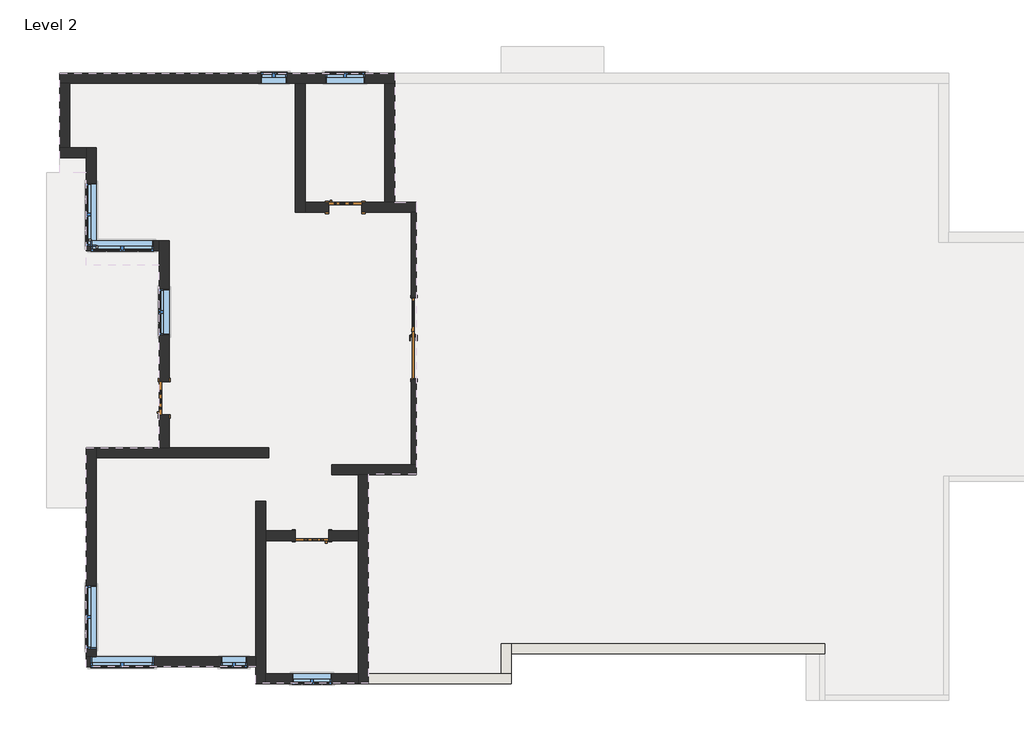
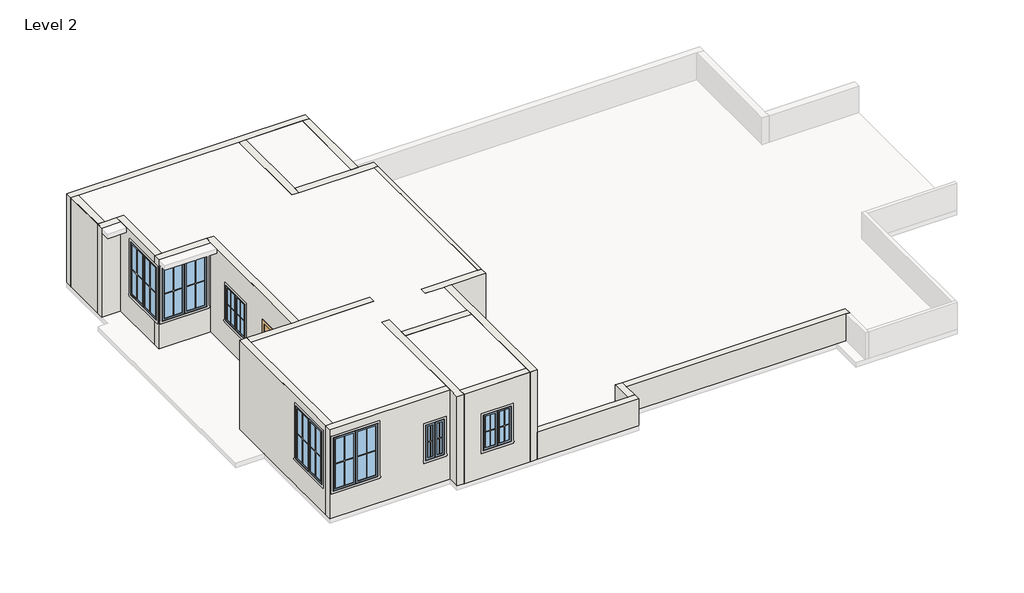
# One storey, part 1 of 2: 21 walls, 9 windows, 4 doors.
"""IFC4 building model written with IfcOpenShell, lengths in millimetres."""

from ifc_helpers import new_model, si_unit, frame, origin, place, context, project, spatial, polyline, outline, extrude, faceted_brep, transform, mapped, element, save
from components import main_entrance_door_11153_main_entrance_door_11153_78fb3b47, door_beb2f668, window_782a76c6, window_d341e8ac, window_2032b2cd, window_9ac97e1a

model = new_model("IFC4")

# Units and contexts
model_context = context("Model", 3, world=origin())
ifc_project = project(units=[si_unit("LENGTHUNIT", "METRE", prefix="MILLI")], contexts=[model_context])

# Site, building, storey
site = spatial("IfcSite", under=ifc_project)
building = spatial("IfcBuilding", under=site)
storey = spatial("IfcBuildingStorey", under=building, Name="Level 2", Elevation=3048.0)

# Doors
placement = place(None, origin())
main_entrance_door_11153_main_entrance_door_11153_shape = main_entrance_door_11153_main_entrance_door_11153_78fb3b47(model_context)
element("IfcDoor", 1, ObjectType="Main_entrance_door_11153 : Main_entrance_door_11153", at=placement, inside=storey, context=model_context, shape_type="MappedRepresentation", body=[
    mapped(main_entrance_door_11153_main_entrance_door_11153_shape, transform((-34548.8645004, 13567.7256148, 3048.0), x_axis=(0.0, 1.0, 0.0), y_axis=(-1.0, 0.0, 0.0), z_axis=(0.0, 0.0, 1.0))),
])
door_shape = door_beb2f668(model_context)
element("IfcDoor", 2, ObjectType="Modern_door_design_10442 : 30\" x 84\"", at=placement, inside=storey, context=model_context, shape_type="MappedRepresentation", body=[
    mapped(door_shape, transform((-36866.6145004, 9033.7472085, 3048.0), x_axis=(-1.0, 0.0, 0.0), y_axis=(0.0, -1.0, 0.0), z_axis=(0.0, 0.0, 1.0))),
])
element("IfcDoor", 3, ObjectType="Modern_door_design_10442 : 30\" x 84\"", at=placement, inside=storey, context=model_context, shape_type="MappedRepresentation", body=[
    mapped(door_shape, transform((-36155.4145004, 16577.6256148, 3048.0), x_axis=(1.0, 0.0, 0.0), y_axis=(0.0, 1.0, 0.0), z_axis=(0.0, 0.0, 1.0))),
])
element("IfcDoor", 4, ObjectType="Modern_door_design_10442 : 30\" x 84\"", at=placement, inside=storey, context=model_context, shape_type="MappedRepresentation", body=[
    mapped(door_shape, transform((-40282.9145004, 12170.804021, 3048.0), x_axis=(0.0, 1.0, 0.0), y_axis=(-1.0, 0.0, 0.0), z_axis=(0.0, 0.0, 1.0))),
])

# Walls
element("IfcWall", 5, ObjectType="wall 4.5", at=placement, inside=storey, context=model_context, shape_type="SweptSolid", body=[
    extrude(outline(polyline([(10672.1256148, 6096.0), (16463.3256148, 6096.0), (16463.3256148, 3048.0), (14517.7256148, 3048.0), (14517.7256148, 5448.0), (12617.7256148, 5448.0), (12617.7256148, 3048.0), (10672.1256148, 3048.0), (10672.1256148, 6096.0)])), frame((-34606.0145004, 0.0, 0.0), z_axis=(1.0, 0.0, 0.0), x_axis=(0.0, 1.0, 0.0)), (0.0, 0.0, 1.0), 114.3),
])
element("IfcWall", 6, ObjectType="wall 9\"", at=placement, inside=storey, context=model_context, shape_type="Brep", body=[
    faceted_brep([(-42683.2145004, 19435.1256148, 3048.0), (-42454.6145004, 19435.1256148, 3048.0), (-37273.0145004, 19435.1256148, 3048.0), (-37044.4145004, 19435.1256148, 3048.0), (-35215.6145004, 19435.1256148, 3048.0), (-34987.0145004, 19435.1256148, 3048.0), (-34987.0145004, 19435.1256148, 3962.4), (-34987.0145004, 19435.1256148, 6096.0), (-35215.6145004, 19435.1256148, 6096.0), (-37044.4145004, 19435.1256148, 6096.0), (-37273.0145004, 19435.1256148, 6096.0), (-42454.6145004, 19435.1256148, 6096.0), (-42683.2145004, 19435.1256148, 6096.0), (-37463.5145004, 19435.1256148, 5181.6), (-37463.5145004, 19435.1256148, 3962.4), (-38073.1145004, 19435.1256148, 3962.4), (-38073.1145004, 19435.1256148, 5181.6), (-35672.8145004, 19435.1256148, 5181.6), (-35672.8145004, 19435.1256148, 3962.4), (-36587.2145004, 19435.1256148, 3962.4), (-36587.2145004, 19435.1256148, 5181.6), (-42683.2145004, 19663.7256148, 3048.0), (-42683.2145004, 19663.7256148, 6096.0), (-34987.0145004, 19663.7256148, 6096.0), (-34987.0145004, 19663.7256148, 3962.4), (-34987.0145004, 19663.7256148, 3048.0), (-37463.5145004, 19663.7256148, 5181.6), (-38073.1145004, 19663.7256148, 5181.6), (-38073.1145004, 19663.7256148, 3962.4), (-37463.5145004, 19663.7256148, 3962.4), (-35672.8145004, 19663.7256148, 5181.6), (-36587.2145004, 19663.7256148, 5181.6), (-36587.2145004, 19663.7256148, 3962.4), (-35672.8145004, 19663.7256148, 3962.4)], [[[0, 1, 2, 3, 4, 5, 6, 7, 8, 9, 10, 11, 12], [13, 14, 15, 16], [17, 18, 19, 20]], [[21, 22, 23, 24, 25], [26, 27, 28, 29], [30, 31, 32, 33]], [[5, 4, 3, 2, 1, 0, 21, 25]], [[12, 11, 10, 9, 8, 7, 23, 22]], [[0, 12, 22, 21]], [[14, 13, 26, 29]], [[15, 14, 29, 28]], [[16, 15, 28, 27]], [[13, 16, 27, 26]], [[18, 17, 30, 33]], [[19, 18, 33, 32]], [[20, 19, 32, 31]], [[17, 20, 31, 30]], [[5, 25, 24, 23, 7, 6]]]),
])
element("IfcWall", 7, ObjectType="wall 9\"", at=placement, inside=storey, context=model_context, shape_type="SweptSolid", body=[
    extrude(outline(polyline([(-35215.6145004, 16691.9256148), (-35215.6145004, 19435.1256148), (-34987.0145004, 19435.1256148), (-34987.0145004, 16691.9256148), (-35215.6145004, 16691.9256148)])), frame((0.0, 0.0, 3048.0), z_axis=(0.0, 0.0, 1.0), x_axis=(1.0, 0.0, 0.0)), (0.0, 0.0, 1.0), 3048.0),
])
element("IfcWall", 8, ObjectType="wall 9\"", at=placement, inside=storey, context=model_context, shape_type="Brep", body=[
    faceted_brep([(-35749.0145004, 16463.3256148, 5181.6), (-35749.0145004, 16463.3256148, 3048.0), (-34606.0145004, 16463.3256148, 3048.0), (-34491.7145004, 16463.3256148, 3048.0), (-34491.7145004, 16463.3256148, 6096.0), (-34606.0145004, 16463.3256148, 6096.0), (-37044.4145004, 16463.3256148, 6096.0), (-37044.4145004, 16463.3256148, 3048.0), (-36511.0145004, 16463.3256148, 3048.0), (-36511.0145004, 16463.3256148, 5181.6), (-34491.7145004, 16691.9256148, 3048.0), (-34987.0145004, 16691.9256148, 3048.0), (-35215.6145004, 16691.9256148, 3048.0), (-35749.0145004, 16691.9256148, 3048.0), (-35749.0145004, 16691.9256148, 5181.6), (-36511.0145004, 16691.9256148, 5181.6), (-36511.0145004, 16691.9256148, 3048.0), (-37044.4145004, 16691.9256148, 3048.0), (-37044.4145004, 16691.9256148, 6096.0), (-35215.6145004, 16691.9256148, 6096.0), (-34987.0145004, 16691.9256148, 6096.0), (-34491.7145004, 16691.9256148, 6096.0)], [[[0, 1, 2, 3, 4, 5, 6, 7, 8, 9]], [[10, 11, 12, 13, 14, 15, 16, 17, 18, 19, 20, 21]], [[8, 7, 17, 16]], [[3, 2, 1, 13, 12, 11, 10]], [[6, 5, 4, 21, 20, 19, 18]], [[7, 6, 18, 17]], [[4, 3, 10, 21]], [[14, 13, 1, 0]], [[15, 14, 0, 9]], [[16, 15, 9, 8]]]),
])
element("IfcWall", 9, ObjectType="wall 9\"", at=placement, inside=storey, context=model_context, shape_type="Brep", body=[
    faceted_brep([(-34491.7145004, 10672.1256148, 3048.0), (-34606.0145004, 10672.1256148, 3048.0), (-36434.8145004, 10672.1256148, 3048.0), (-36434.8145004, 10672.1256148, 6096.0), (-34606.0145004, 10672.1256148, 6096.0), (-34491.7145004, 10672.1256148, 6096.0), (-34491.7145004, 10443.5256148, 3048.0), (-34491.7145004, 10443.5256148, 6096.0), (-35596.6145004, 10443.5256148, 6096.0), (-35825.2145004, 10443.5256148, 6096.0), (-36434.8145004, 10443.5256148, 6096.0), (-36434.8145004, 10443.5256148, 3048.0), (-35825.2145004, 10443.5256148, 3048.0), (-35596.6145004, 10443.5256148, 3048.0)], [[[0, 1, 2, 3, 4, 5]], [[6, 7, 8, 9, 10, 11, 12, 13]], [[2, 1, 0, 6, 13, 12, 11]], [[3, 2, 11, 10]], [[5, 4, 3, 10, 9, 8, 7]], [[0, 5, 7, 6]]]),
])
element("IfcWall", 10, ObjectType="wall 9\"", at=placement, inside=storey, context=model_context, shape_type="Brep", body=[
    faceted_brep([(-35825.2145004, 10443.5256148, 3048.0), (-35825.2145004, 9148.0472085, 3048.0), (-35825.2145004, 8919.4472085, 3048.0), (-35825.2145004, 5871.4472085, 3048.0), (-35825.2145004, 5642.8472085, 3048.0), (-35825.2145004, 5642.8472085, 6096.0), (-35825.2145004, 5871.4472085, 6096.0), (-35825.2145004, 8919.4472085, 6096.0), (-35825.2145004, 9148.0472085, 6096.0), (-35825.2145004, 10443.5256148, 6096.0), (-35596.6145004, 10443.5256148, 3048.0), (-35596.6145004, 10443.5256148, 6096.0), (-35596.6145004, 5642.8472085, 6096.0), (-35596.6145004, 5642.8472085, 3962.4), (-35596.6145004, 5642.8472085, 3048.0), (-35596.6145004, 5871.4472085, 3048.0)], [[[0, 1, 2, 3, 4, 5, 6, 7, 8, 9]], [[10, 11, 12, 13, 14, 15]], [[4, 3, 2, 1, 0, 10, 15, 14]], [[9, 8, 7, 6, 5, 12, 11]], [[0, 9, 11, 10]], [[4, 14, 13, 12, 5]]]),
])
element("IfcWall", 11, ObjectType="wall 9\"", at=placement, inside=storey, context=model_context, shape_type="SweptSolid", body=[
    extrude(outline(polyline([(3048.0, -35825.2145004), (6096.0, -35825.2145004), (6096.0, -37958.8145004), (3048.0, -37958.8145004), (3048.0, -35825.2145004)]), holes=[polyline([(5181.6, -37349.2145004), (5181.6, -36434.8145004), (3962.4, -36434.8145004), (3962.4, -37349.2145004), (5181.6, -37349.2145004)])]), frame((0.0, 5642.8472085, 0.0), z_axis=(0.0, 1.0, 0.0), x_axis=(0.0, 0.0, 1.0)), (0.0, 0.0, 1.0), 228.6),
])
element("IfcWall", 12, ObjectType="wall 9\"", at=placement, inside=storey, context=model_context, shape_type="Brep", body=[
    faceted_brep([(-37958.8145004, 5642.8472085, 3048.0), (-37958.8145004, 5871.4472085, 3048.0), (-37958.8145004, 8919.4472085, 3048.0), (-37958.8145004, 9148.0472085, 3048.0), (-37958.8145004, 9833.9256148, 3048.0), (-37958.8145004, 9833.9256148, 6096.0), (-37958.8145004, 9148.0472085, 6096.0), (-37958.8145004, 8919.4472085, 6096.0), (-37958.8145004, 5871.4472085, 6096.0), (-37958.8145004, 5642.8472085, 6096.0), (-38187.4145004, 5642.8472085, 3048.0), (-38187.4145004, 5642.8472085, 6096.0), (-38187.4145004, 6023.9256148, 6096.0), (-38187.4145004, 6252.5256148, 6096.0), (-38187.4145004, 9833.9256148, 6096.0), (-38187.4145004, 9833.9256148, 3048.0), (-38187.4145004, 6252.5256148, 3048.0), (-38187.4145004, 6023.9256148, 3048.0)], [[[0, 1, 2, 3, 4, 5, 6, 7, 8, 9]], [[10, 11, 12, 13, 14, 15, 16, 17]], [[4, 3, 2, 1, 0, 10, 17, 16, 15]], [[5, 4, 15, 14]], [[9, 8, 7, 6, 5, 14, 13, 12, 11]], [[0, 9, 11, 10]]]),
])
element("IfcWall", 13, ObjectType="wall 9\"", at=placement, inside=storey, context=model_context, shape_type="Brep", body=[
    faceted_brep([(-38187.4145004, 6252.5256148, 3048.0), (-41845.0145004, 6252.5256148, 3048.0), (-42073.6145004, 6252.5256148, 3048.0), (-42073.6145004, 6252.5256148, 6096.0), (-41845.0145004, 6252.5256148, 6096.0), (-38187.4145004, 6252.5256148, 6096.0), (-38987.5145004, 6252.5256148, 5181.6), (-38987.5145004, 6252.5256148, 3962.4), (-38377.9145004, 6252.5256148, 3962.4), (-38377.9145004, 6252.5256148, 5181.6), (-41972.0145004, 6252.5256148, 5791.2), (-41972.0145004, 6252.5256148, 3962.4), (-40524.2145004, 6252.5256148, 3962.4), (-40524.2145004, 6252.5256148, 5791.2), (-38187.4145004, 6023.9256148, 3048.0), (-38187.4145004, 6023.9256148, 6096.0), (-42073.6145004, 6023.9256148, 6096.0), (-42073.6145004, 6023.9256148, 3048.0), (-38987.5145004, 6023.9256148, 5181.6), (-38377.9145004, 6023.9256148, 5181.6), (-38377.9145004, 6023.9256148, 3962.4), (-38987.5145004, 6023.9256148, 3962.4), (-41972.0145004, 6023.9256148, 5791.2), (-40524.2145004, 6023.9256148, 5791.2), (-40524.2145004, 6023.9256148, 3962.4), (-41972.0145004, 6023.9256148, 3962.4)], [[[0, 1, 2, 3, 4, 5], [6, 7, 8, 9], [10, 11, 12, 13]], [[14, 15, 16, 17], [18, 19, 20, 21], [22, 23, 24, 25]], [[2, 1, 0, 14, 17]], [[5, 4, 3, 16, 15]], [[0, 5, 15, 14]], [[3, 2, 17, 16]], [[7, 6, 18, 21]], [[8, 7, 21, 20]], [[9, 8, 20, 19]], [[6, 9, 19, 18]], [[11, 10, 22, 25]], [[12, 11, 25, 24]], [[13, 12, 24, 23]], [[10, 13, 23, 22]]]),
])
element("IfcWall", 14, ObjectType="wall 9\"", at=placement, inside=storey, context=model_context, shape_type="Brep", body=[
    faceted_brep([(-41845.0145004, 6252.5256148, 3048.0), (-41845.0145004, 10824.5256148, 3048.0), (-41845.0145004, 11053.1256148, 3048.0), (-41845.0145004, 11053.1256148, 6096.0), (-41845.0145004, 10824.5256148, 6096.0), (-41845.0145004, 6252.5256148, 6096.0), (-41845.0145004, 7890.904021, 5791.2), (-41845.0145004, 7890.904021, 3962.4), (-41845.0145004, 6443.104021, 3962.4), (-41845.0145004, 6443.104021, 5791.2), (-42073.6145004, 11053.1256148, 3048.0), (-42073.6145004, 6252.5256148, 3048.0), (-42073.6145004, 6252.5256148, 6096.0), (-42073.6145004, 11053.1256148, 6096.0), (-42073.6145004, 7890.904021, 3962.4), (-42073.6145004, 7890.904021, 5791.2), (-42073.6145004, 6443.104021, 5791.2), (-42073.6145004, 6443.104021, 3962.4)], [[[0, 1, 2, 3, 4, 5], [6, 7, 8, 9]], [[10, 11, 12, 13], [14, 15, 16, 17]], [[2, 1, 0, 11, 10]], [[5, 4, 3, 13, 12]], [[0, 5, 12, 11]], [[3, 2, 10, 13]], [[6, 15, 14, 7]], [[7, 14, 17, 8]], [[15, 6, 9, 16]], [[16, 9, 8, 17]]]),
])
element("IfcWall", 15, ObjectType="wall 9\"", at=placement, inside=storey, context=model_context, shape_type="Brep", body=[
    faceted_brep([(-41845.0145004, 10824.5256148, 3048.0), (-37882.6145004, 10824.5256148, 3048.0), (-37882.6145004, 10824.5256148, 6096.0), (-41845.0145004, 10824.5256148, 6096.0), (-41845.0145004, 11053.1256148, 3048.0), (-41845.0145004, 11053.1256148, 6096.0), (-40397.2145004, 11053.1256148, 6096.0), (-40168.6145004, 11053.1256148, 6096.0), (-37882.6145004, 11053.1256148, 6096.0), (-37882.6145004, 11053.1256148, 3048.0), (-40168.6145004, 11053.1256148, 3048.0), (-40397.2145004, 11053.1256148, 3048.0)], [[[0, 1, 2, 3]], [[4, 5, 6, 7, 8, 9, 10, 11]], [[1, 0, 4, 11, 10, 9]], [[2, 1, 9, 8]], [[3, 2, 8, 7, 6, 5]], [[0, 3, 5, 4]]]),
])
element("IfcWall", 16, ObjectType="wall 9\"", at=placement, inside=storey, context=model_context, shape_type="Brep", body=[
    faceted_brep([(-40168.6145004, 12577.204021, 5181.6), (-40168.6145004, 12577.204021, 3048.0), (-40168.6145004, 15815.704021, 3048.0), (-40168.6145004, 15815.704021, 6096.0), (-40168.6145004, 11053.1256148, 6096.0), (-40168.6145004, 11053.1256148, 3048.0), (-40168.6145004, 11815.204021, 3048.0), (-40168.6145004, 11815.204021, 5181.6), (-40168.6145004, 14710.804021, 5181.6), (-40168.6145004, 14710.804021, 3962.4), (-40168.6145004, 13644.004021, 3962.4), (-40168.6145004, 13644.004021, 5181.6), (-40397.2145004, 15815.704021, 3048.0), (-40397.2145004, 15587.104021, 3048.0), (-40397.2145004, 12577.204021, 3048.0), (-40397.2145004, 12577.204021, 5181.6), (-40397.2145004, 11815.204021, 5181.6), (-40397.2145004, 11815.204021, 3048.0), (-40397.2145004, 11053.1256148, 3048.0), (-40397.2145004, 11053.1256148, 6096.0), (-40397.2145004, 15587.104021, 6096.0), (-40397.2145004, 15815.704021, 6096.0), (-40397.2145004, 14710.804021, 5181.6), (-40397.2145004, 13644.004021, 5181.6), (-40397.2145004, 13644.004021, 3962.4), (-40397.2145004, 14710.804021, 3962.4)], [[[0, 1, 2, 3, 4, 5, 6, 7], [8, 9, 10, 11]], [[12, 13, 14, 15, 16, 17, 18, 19, 20, 21], [22, 23, 24, 25]], [[6, 5, 18, 17]], [[2, 1, 14, 13, 12]], [[4, 3, 21, 20, 19]], [[5, 4, 19, 18]], [[3, 2, 12, 21]], [[15, 14, 1, 0]], [[16, 15, 0, 7]], [[17, 16, 7, 6]], [[9, 8, 22, 25]], [[10, 9, 25, 24]], [[11, 10, 24, 23]], [[8, 11, 23, 22]]]),
])
element("IfcWall", 17, ObjectType="wall 9\"", at=placement, inside=storey, context=model_context, shape_type="Brep", body=[
    faceted_brep([(-40397.2145004, 15815.704021, 3048.0), (-41845.0145004, 15815.704021, 3048.0), (-42073.6145004, 15815.704021, 3048.0), (-42073.6145004, 15815.704021, 3962.4), (-41845.0145004, 15815.704021, 3962.4), (-40524.2145004, 15815.704021, 3962.4), (-40524.2145004, 15815.704021, 5791.2), (-41845.0145004, 15815.704021, 5791.2), (-42073.6145004, 15815.704021, 5791.2), (-42073.6145004, 15815.704021, 6096.0), (-41845.0145004, 15815.704021, 6096.0), (-40397.2145004, 15815.704021, 6096.0), (-42073.6145004, 15587.104021, 3048.0), (-40397.2145004, 15587.104021, 3048.0), (-40397.2145004, 15587.104021, 6096.0), (-42073.6145004, 15587.104021, 6096.0), (-41972.0145004, 15587.104021, 3962.4), (-41972.0145004, 15587.104021, 5791.2), (-40524.2145004, 15587.104021, 5791.2), (-40524.2145004, 15587.104021, 3962.4), (-42073.6145004, 15688.704021, 5791.2), (-42073.6145004, 15688.704021, 3962.4), (-41972.0145004, 15688.704021, 3962.4), (-41972.0145004, 15688.704021, 5791.2)], [[[0, 1, 2, 3, 4, 5, 6, 7, 8, 9, 10, 11]], [[12, 13, 14, 15], [16, 17, 18, 19]], [[2, 1, 0, 13, 12]], [[11, 10, 9, 15, 14]], [[0, 11, 14, 13]], [[2, 12, 15, 9, 8, 20, 21, 3]], [[17, 16, 22, 23]], [[16, 19, 5, 4, 3, 21, 22]], [[6, 5, 19, 18]], [[18, 17, 23, 20, 8, 7, 6]], [[20, 23, 22, 21]]]),
])
element("IfcWall", 18, ObjectType="wall 9\"", at=placement, inside=storey, context=model_context, shape_type="Brep", body=[
    faceted_brep([(-41845.0145004, 15815.704021, 3048.0), (-41845.0145004, 17949.304021, 3048.0), (-41845.0145004, 17949.304021, 6096.0), (-41845.0145004, 15815.704021, 6096.0), (-41845.0145004, 15815.704021, 5791.2), (-41845.0145004, 17136.504021, 5791.2), (-41845.0145004, 17136.504021, 3962.4), (-41845.0145004, 15815.704021, 3962.4), (-42073.6145004, 17949.304021, 3048.0), (-42073.6145004, 17720.704021, 3048.0), (-42073.6145004, 15815.704021, 3048.0), (-42073.6145004, 15815.704021, 3962.4), (-42073.6145004, 17136.504021, 3962.4), (-42073.6145004, 17136.504021, 5791.2), (-42073.6145004, 15815.704021, 5791.2), (-42073.6145004, 15815.704021, 6096.0), (-42073.6145004, 17720.704021, 6096.0), (-42073.6145004, 17949.304021, 6096.0)], [[[0, 1, 2, 3, 4, 5, 6, 7]], [[8, 9, 10, 11, 12, 13, 14, 15, 16, 17]], [[1, 0, 10, 9, 8]], [[3, 2, 17, 16, 15]], [[3, 15, 14, 4]], [[10, 0, 7, 11]], [[2, 1, 8, 17]], [[5, 13, 12, 6]], [[6, 12, 11, 7]], [[13, 5, 4, 14]]]),
])
element("IfcWall", 19, ObjectType="wall 9\"", at=placement, inside=storey, context=model_context, shape_type="Brep", body=[
    faceted_brep([(-42073.6145004, 17949.304021, 3048.0), (-42454.6145004, 17949.304021, 3048.0), (-42683.2145004, 17949.304021, 3048.0), (-42683.2145004, 17949.304021, 6096.0), (-42454.6145004, 17949.304021, 6096.0), (-42073.6145004, 17949.304021, 6096.0), (-42073.6145004, 17720.704021, 3048.0), (-42073.6145004, 17720.704021, 6096.0), (-42683.2145004, 17720.704021, 6096.0), (-42683.2145004, 17720.704021, 3048.0)], [[[0, 1, 2, 3, 4, 5]], [[6, 7, 8, 9]], [[2, 1, 0, 6, 9]], [[5, 4, 3, 8, 7]], [[0, 5, 7, 6]], [[3, 2, 9, 8]]]),
])
element("IfcWall", 20, ObjectType="wall 9\"", at=placement, inside=storey, context=model_context, shape_type="SweptSolid", body=[
    extrude(outline(polyline([(-42683.2145004, 17949.304021), (-42683.2145004, 19435.1256148), (-42454.6145004, 19435.1256148), (-42454.6145004, 17949.304021), (-42683.2145004, 17949.304021)])), frame((0.0, 0.0, 3048.0), z_axis=(0.0, 0.0, 1.0), x_axis=(1.0, 0.0, 0.0)), (0.0, 0.0, 1.0), 3048.0),
])
element("IfcWall", 21, ObjectType="wall 9\"", at=placement, inside=storey, context=model_context, shape_type="Brep", body=[
    faceted_brep([(-37273.0145004, 19435.1256148, 3048.0), (-37273.0145004, 16463.3256148, 3048.0), (-37273.0145004, 16463.3256148, 6096.0), (-37273.0145004, 19435.1256148, 6096.0), (-37044.4145004, 19435.1256148, 3048.0), (-37044.4145004, 19435.1256148, 6096.0), (-37044.4145004, 16691.9256148, 6096.0), (-37044.4145004, 16463.3256148, 6096.0), (-37044.4145004, 16463.3256148, 3048.0), (-37044.4145004, 16691.9256148, 3048.0)], [[[0, 1, 2, 3]], [[4, 5, 6, 7, 8, 9]], [[1, 0, 4, 9, 8]], [[3, 2, 7, 6, 5]], [[0, 3, 5, 4]], [[2, 1, 8, 7]]]),
])
element("IfcWall", 22, ObjectType="wall 9\"", at=placement, inside=storey, context=model_context, shape_type="SweptSolid", body=[
    extrude(outline(polyline([(3048.0, -37958.8145004), (3048.0, -37273.0145004), (5181.6, -37273.0145004), (5181.6, -36511.0145004), (3048.0, -36511.0145004), (3048.0, -35825.2145004), (6096.0, -35825.2145004), (6096.0, -37958.8145004), (3048.0, -37958.8145004)])), frame((0.0, 8919.4472085, 0.0), z_axis=(0.0, 1.0, 0.0), x_axis=(0.0, 0.0, 1.0)), (0.0, 0.0, 1.0), 228.6),
])
element("IfcWall", 23, ObjectType="wall 9\"", at=placement, inside=storey, context=model_context, shape_type="Brep", body=[
    faceted_brep([(-35596.6145004, 5642.8472085, 3048.0), (-32320.0145004, 5642.8472085, 3048.0), (-32320.0145004, 5642.8472085, 3962.4), (-35596.6145004, 5642.8472085, 3962.4), (-35596.6145004, 5871.4472085, 3048.0), (-35596.6145004, 5871.4472085, 3962.4), (-32548.6145004, 5871.4472085, 3962.4), (-32320.0145004, 5871.4472085, 3962.4), (-32320.0145004, 5871.4472085, 3048.0), (-32548.6145004, 5871.4472085, 3048.0)], [[[0, 1, 2, 3]], [[4, 5, 6, 7, 8, 9]], [[1, 0, 4, 9, 8]], [[3, 2, 7, 6, 5]], [[2, 1, 8, 7]], [[0, 3, 5, 4]]]),
])
element("IfcWall", 24, ObjectType="wall 9\"", at=placement, inside=storey, context=model_context, shape_type="Brep", body=[
    faceted_brep([(-32320.0145004, 5871.4472085, 3048.0), (-32320.0145004, 6328.7256148, 3048.0), (-32320.0145004, 6557.3256148, 3048.0), (-32320.0145004, 6557.3256148, 3962.4), (-32320.0145004, 6328.7256148, 3962.4), (-32320.0145004, 5871.4472085, 3962.4), (-32548.6145004, 5871.4472085, 3048.0), (-32548.6145004, 5871.4472085, 3962.4), (-32548.6145004, 6557.3256148, 3962.4), (-32548.6145004, 6557.3256148, 3048.0)], [[[0, 1, 2, 3, 4, 5]], [[6, 7, 8, 9]], [[2, 1, 0, 6, 9]], [[5, 4, 3, 8, 7]], [[0, 5, 7, 6]], [[3, 2, 9, 8]]]),
])
element("IfcWall", 25, ObjectType="wall 9\"", at=placement, inside=storey, context=model_context, shape_type="Brep", body=[
    faceted_brep([(-32320.0145004, 6328.7256148, 3048.0), (-25233.4145004, 6328.7256148, 3048.0), (-25119.1145004, 6328.7256148, 3048.0), (-25119.1145004, 6328.7256148, 3962.4), (-25233.4145004, 6328.7256148, 3962.4), (-32320.0145004, 6328.7256148, 3962.4), (-32320.0145004, 6557.3256148, 3048.0), (-32320.0145004, 6557.3256148, 3962.4), (-25119.1145004, 6557.3256148, 3962.4), (-25119.1145004, 6557.3256148, 3048.0)], [[[0, 1, 2, 3, 4, 5]], [[6, 7, 8, 9]], [[2, 1, 0, 6, 9]], [[5, 4, 3, 8, 7]], [[0, 5, 7, 6]], [[3, 2, 9, 8]]]),
])

# Windows
window_shape = window_782a76c6(model_context)
element("IfcWindow", 26, ObjectType="Window-Casement-Double : 24\"X48\"", at=placement, inside=storey, context=model_context, shape_type="MappedRepresentation", body=[
    mapped(window_shape, transform((-38682.7145004, 6138.2256148, 3048.0), x_axis=(-1.0, 0.0, 0.0), y_axis=(0.0, -1.0, 0.0), z_axis=(0.0, 0.0, 1.0))),
])
element("IfcWindow", 27, ObjectType="Window-Casement-Double : 24\"X48\"", at=placement, inside=storey, context=model_context, shape_type="MappedRepresentation", body=[
    mapped(window_shape, transform((-37768.3145004, 19549.4256148, 3048.0), x_axis=(1.0, 0.0, 0.0), y_axis=(0.0, 1.0, 0.0), z_axis=(0.0, 0.0, 1.0))),
])
window_2_shape = window_d341e8ac(model_context)
element("IfcWindow", 28, ObjectType="Window-Casement-Double : 36\"X48\"", at=placement, inside=storey, context=model_context, shape_type="MappedRepresentation", body=[
    mapped(window_2_shape, transform((-36130.0145004, 19549.4256148, 3048.0), x_axis=(1.0, 0.0, 0.0), y_axis=(0.0, 1.0, 0.0), z_axis=(0.0, 0.0, 1.0))),
])
element("IfcWindow", 29, ObjectType="Window-Casement-Double : 36\"X48\"", at=placement, inside=storey, context=model_context, shape_type="MappedRepresentation", body=[
    mapped(window_2_shape, transform((-36892.0145004, 5757.1472085, 3048.0), x_axis=(-1.0, 0.0, 0.0), y_axis=(0.0, -1.0, 0.0), z_axis=(0.0, 0.0, 1.0))),
])
window_3_shape = window_2032b2cd(model_context)
element("IfcWindow", 30, ObjectType="Window-Casement-Double : 42\"X48\"", at=placement, inside=storey, context=model_context, shape_type="MappedRepresentation", body=[
    mapped(window_3_shape, transform((-40282.9145004, 14177.404021, 3048.0), x_axis=(0.0, 1.0, 0.0), y_axis=(-1.0, 0.0, 0.0), z_axis=(0.0, 0.0, 1.0))),
])
window_4_shape = window_9ac97e1a(model_context)
element("IfcWindow", 31, ObjectType="Window-Casement-Double : 57\" x 72\"", at=placement, inside=storey, context=model_context, shape_type="MappedRepresentation", body=[
    mapped(window_4_shape, transform((-41248.1145004, 6138.2256148, 3048.0), x_axis=(-1.0, 0.0, 0.0), y_axis=(0.0, -1.0, 0.0), z_axis=(0.0, 0.0, 1.0))),
])
element("IfcWindow", 32, ObjectType="Window-Casement-Double : 57\" x 72\"", at=placement, inside=storey, context=model_context, shape_type="MappedRepresentation", body=[
    mapped(window_4_shape, transform((-41959.3145004, 7167.004021, 3048.0), x_axis=(0.0, 1.0, 0.0), y_axis=(-1.0, 0.0, 0.0), z_axis=(0.0, 0.0, 1.0))),
])
element("IfcWindow", 33, ObjectType="Window-Casement-Double : 57\" x 72\"", at=placement, inside=storey, context=model_context, shape_type="MappedRepresentation", body=[
    mapped(window_4_shape, transform((-41248.1145004, 15701.404021, 3048.0), x_axis=(-1.0, 0.0, 0.0), y_axis=(0.0, -1.0, 0.0), z_axis=(0.0, 0.0, 1.0))),
])
element("IfcWindow", 34, ObjectType="Window-Casement-Double : 57\" x 72\"", at=placement, inside=storey, context=model_context, shape_type="MappedRepresentation", body=[
    mapped(window_4_shape, transform((-41959.3145004, 16412.604021, 3048.0), x_axis=(0.0, 1.0, 0.0), y_axis=(-1.0, 0.0, 0.0), z_axis=(0.0, 0.0, 1.0))),
])

save(model, "model.ifc")

# Revit data of these elements
# Type "Main_entrance_door_11153 : Main_entrance_door_11153"
#   Type Mark = "22"
#   Height = 7' - 10.48819"
#   Width = 6' - 2.80315"
#   Door Width = 3' - 7.30709"
#   Function = (empty or 0)
#   Wall Closure = (empty or 0)
# Type "Modern_door_design_10442 : 30\" x 84\""
#   Type Mark = "18"
#   Assembly Code = "C1020"
#   Thickness = 0' - 2"
#   Height = 7' - 0"
#   Muntin = 0' - 1"
#   Stile Width = 0' - 5"
#   Trim Projection Ext = 0' - 1"
#   Trim Projection Int = 0' - 1"
#   Trim Width = 0' - 3"
#   Width = 2' - 6"
#   Door Material = Door - Panel
#   Frame Material = Door - Frame
#   Function = (empty or 0)
#   Wall Closure = (empty or 0)
# Type "wall 4.5"
#   Assembly Code = "B2010"
#   Layers, outside or top first: 0' - 4 1/2" no material (function 1)
# Type "wall 9\""
#   Assembly Code = "B2010"
#   Layers, outside or top first: 0' - 9" no material (function 1)
# Type "Window-Casement-Double : 24\"X48\""
#   Type Mark = "22"
#   Fire Rating = "0.5h"
#   Assembly Code = "B2020100"
#   Analytic Construction = "Double glazing - domestic"
#   Frame Extension [instance default] = 0' - 0 1/4"
#   Window Inset [instance default] = 0' - 0"
#   Wall Thickness [instance default] = 0' - 6"
#   Interior Wall Closure [instance default] = 0' - 2 1/4"
#   Half Width = 1' - 0"
#   Visual Light Transmittance = 0.81
#   Thermal Resistance (R) = 1.8146 (h·ft²·°F)/BTU
#   Solar Heat Gain Coefficient = 0.76
#   Rough Width = 2' - 0 1/2"
#   Rough Height = 4' - 0 1/2"
#   Height = 4' - 0"
#   Heat Transfer Coefficient (U) = 0.5511 BTU/(h·ft²·°F)
#   Exterior Wall Closure [instance default] = 0' - 1 1/4"
#   Extension Jamb [instance default] = 0' - 2 1/4"
#   Default Sill Height = 3' - 0"
#   Width = 2' - 0"
#   Muntin Visibility = yes
#   Interior Trim Visibility [instance default] = yes
#   Exterior Trim Visibility [instance default] = yes
#   Extension Jamb Visibility [instance default] = yes
#   Interior Trim Material = Wood - Stained
#   Muntin Pattern = Muntin Pattern_2x2 : Muntin Pattern_2x2
#   Interior Trim = Trim-Window-Interior-Flat : Picture Frame
#   Interior Frame Material = Wood - Stained
#   Glass Panel Material = Glass
#   Exterior Trim Material = Clad - White
#   Exterior Trim = Trim-Window-Exterior-Flat : with Sill
#   Exterior Frame Material = Clad - White
#   Wall Closure = (empty or 0)
# Type "Window-Casement-Double : 36\"X48\""
#   Type Mark = "21"
#   Fire Rating = "0.5h"
#   Assembly Code = "B2020100"
#   Analytic Construction = "Double glazing - domestic"
#   Frame Extension [instance default] = 0' - 0 1/4"
#   Window Inset [instance default] = 0' - 0"
#   Wall Thickness [instance default] = 0' - 6"
#   Interior Wall Closure [instance default] = 0' - 2 1/4"
#   Half Width = 1' - 6"
#   Visual Light Transmittance = 0.81
#   Thermal Resistance (R) = 1.8146 (h·ft²·°F)/BTU
#   Solar Heat Gain Coefficient = 0.76
#   Rough Width = 3' - 0 1/2"
#   Rough Height = 4' - 0 1/2"
#   Height = 4' - 0"
#   Heat Transfer Coefficient (U) = 0.5511 BTU/(h·ft²·°F)
#   Exterior Wall Closure [instance default] = 0' - 1 1/4"
#   Extension Jamb [instance default] = 0' - 2 1/4"
#   Default Sill Height = 3' - 0"
#   Width = 3' - 0"
#   Muntin Visibility = yes
#   Interior Trim Visibility [instance default] = yes
#   Exterior Trim Visibility [instance default] = yes
#   Extension Jamb Visibility [instance default] = yes
#   Interior Trim Material = Wood - Stained
#   Muntin Pattern = Muntin Pattern_2x2 : Muntin Pattern_2x2
#   Interior Trim = Trim-Window-Interior-Flat : Picture Frame
#   Interior Frame Material = Wood - Stained
#   Glass Panel Material = Glass
#   Exterior Trim Material = Clad - White
#   Exterior Trim = Trim-Window-Exterior-Flat : with Sill
#   Exterior Frame Material = Clad - White
#   Wall Closure = (empty or 0)
# Type "Window-Casement-Double : 42\"X48\""
#   Type Mark = "27"
#   Fire Rating = "0.5h"
#   Assembly Code = "B2020100"
#   Analytic Construction = "Double glazing - domestic"
#   Frame Extension [instance default] = 0' - 0 1/4"
#   Window Inset [instance default] = 0' - 0"
#   Wall Thickness [instance default] = 0' - 6"
#   Interior Wall Closure [instance default] = 0' - 2 1/4"
#   Half Width = 1' - 9"
#   Visual Light Transmittance = 0.81
#   Thermal Resistance (R) = 1.8146 (h·ft²·°F)/BTU
#   Solar Heat Gain Coefficient = 0.76
#   Rough Width = 3' - 6 1/2"
#   Rough Height = 4' - 0 1/2"
#   Height = 4' - 0"
#   Heat Transfer Coefficient (U) = 0.5511 BTU/(h·ft²·°F)
#   Exterior Wall Closure [instance default] = 0' - 1 1/4"
#   Extension Jamb [instance default] = 0' - 2 1/4"
#   Default Sill Height = 3' - 0"
#   Width = 3' - 6"
#   Muntin Visibility = yes
#   Interior Trim Visibility [instance default] = yes
#   Exterior Trim Visibility [instance default] = yes
#   Extension Jamb Visibility [instance default] = yes
#   Interior Trim Material = Wood - Stained
#   Muntin Pattern = Muntin Pattern_2x2 : Muntin Pattern_2x2
#   Interior Trim = Trim-Window-Interior-Flat : Picture Frame
#   Interior Frame Material = Wood - Stained
#   Glass Panel Material = Glass
#   Exterior Trim Material = Clad - White
#   Exterior Trim = Trim-Window-Exterior-Flat : with Sill
#   Exterior Frame Material = Clad - White
#   Wall Closure = (empty or 0)
# Type "Window-Casement-Double : 57\" x 72\""
#   Type Mark = "17"
#   Fire Rating = "0.5h"
#   Assembly Code = "B2020100"
#   Analytic Construction = "Double glazing - domestic"
#   Frame Extension [instance default] = 0' - 0 1/4"
#   Window Inset [instance default] = 0' - 0"
#   Wall Thickness [instance default] = 0' - 6"
#   Interior Wall Closure [instance default] = 0' - 2 1/4"
#   Half Width = 2' - 4 1/2"
#   Visual Light Transmittance = 0.81
#   Thermal Resistance (R) = 1.8146 (h·ft²·°F)/BTU
#   Solar Heat Gain Coefficient = 0.76
#   Rough Width = 4' - 9 1/2"
#   Rough Height = 6' - 0 1/2"
#   Height = 6' - 0"
#   Heat Transfer Coefficient (U) = 0.5511 BTU/(h·ft²·°F)
#   Exterior Wall Closure [instance default] = 0' - 1 1/4"
#   Extension Jamb [instance default] = 0' - 2 1/4"
#   Default Sill Height = 3' - 0"
#   Width = 4' - 9"
#   Define Thermal Properties by = 0
#   Muntin Visibility = yes
#   Interior Trim Visibility [instance default] = yes
#   Exterior Trim Visibility [instance default] = yes
#   Extension Jamb Visibility [instance default] = yes
#   Interior Trim Material = Wood - Stained
#   Muntin Pattern = Muntin Pattern_2x2 : Muntin Pattern_2x2
#   Interior Trim = Trim-Window-Interior-Flat : Picture Frame
#   Interior Frame Material = Wood - Stained
#   Glass Panel Material = Glass
#   Exterior Trim Material = Clad - White
#   Exterior Trim = Trim-Window-Exterior-Flat : with Sill
#   Exterior Frame Material = Clad - White
#   Wall Closure = (empty or 0)
# Element 1 (IfcDoor, "Main_entrance_door_11153 : Main_entrance_door_11153")
#   Phase Created = New Construction
#   Materials on its faces: "Glass", "Default"
# Elements 2, 3, 4 (IfcDoor, "Modern_door_design_10442 : 30\" x 84\"")
#   Phase Created = New Construction
#   Materials on its faces: "Door - Frame", "Door - Panel", "Glass", "Door - Handle"
# Element 5 (IfcWall, "wall 4.5")
#   Top Offset = 0' - 0"
#   Base Offset = 0' - 0"
#   wall height = 10' - 0"
#   Phase Created = New Construction
#   Base Constraint = Level 2
#   Top Constraint = Level 3
#   Materials on its faces: "Default Wall"
# Elements 6, 7, 8, 9, 10, 11, 12, 13, 14, 15, 16, 17, 18, 19, 20, 21, 22 (IfcWall, "wall 9\"")
#   Top Offset = 0' - 0"
#   Base Offset = 0' - 0"
#   wall height = 10' - 0"
#   Phase Created = New Construction
#   Base Constraint = Level 2
#   Top Constraint = Level 3
#   Materials on its faces: "Default Wall"
# Elements 23, 24, 25 (IfcWall, "wall 9\"")
#   Top Offset = 0' - 0"
#   Base Offset = 0' - 0"
#   wall height = 3' - 0"
#   Phase Created = New Construction
#   Base Constraint = Level 2
#   Top Constraint = Level 8
#   Materials on its faces: "Default Wall"
# Element 26 (IfcWindow, "Window-Casement-Double : 24\"X48\"")
#   Mark = "34"
#   Window Inset = 0' - 0"
#   Interior Wall Closure = 0' - 2 1/4"
#   Frame Extension = 0' - 0 1/4"
#   Exterior Wall Closure = 0' - 1 1/4"
#   Interior Trim Visibility = yes
#   Exterior Trim Visibility = yes
#   Phase Created = New Construction
#   Materials on its faces: "Wood - Stained", "Glass", "Clad - White"
# Element 27 (IfcWindow, "Window-Casement-Double : 24\"X48\"")
#   Mark = "35"
#   Window Inset = 0' - 0"
#   Interior Wall Closure = 0' - 2 1/4"
#   Frame Extension = 0' - 0 1/4"
#   Exterior Wall Closure = 0' - 1 1/4"
#   Interior Trim Visibility = yes
#   Exterior Trim Visibility = yes
#   Phase Created = New Construction
#   Materials on its faces: "Wood - Stained", "Glass", "Clad - White"
# Element 28 (IfcWindow, "Window-Casement-Double : 36\"X48\"")
#   Mark = "36"
#   Window Inset = 0' - 0"
#   Interior Wall Closure = 0' - 2 1/4"
#   Frame Extension = 0' - 0 1/4"
#   Exterior Wall Closure = 0' - 1 1/4"
#   Interior Trim Visibility = yes
#   Exterior Trim Visibility = yes
#   Phase Created = New Construction
#   Materials on its faces: "Wood - Stained", "Glass", "Clad - White"
# Element 29 (IfcWindow, "Window-Casement-Double : 36\"X48\"")
#   Mark = "37"
#   Window Inset = 0' - 0"
#   Interior Wall Closure = 0' - 2 1/4"
#   Frame Extension = 0' - 0 1/4"
#   Exterior Wall Closure = 0' - 1 1/4"
#   Interior Trim Visibility = yes
#   Exterior Trim Visibility = yes
#   Phase Created = New Construction
#   Materials on its faces: "Wood - Stained", "Glass", "Clad - White"
# Element 30 (IfcWindow, "Window-Casement-Double : 42\"X48\"")
#   Mark = "38"
#   Window Inset = 0' - 0"
#   Interior Wall Closure = 0' - 2 1/4"
#   Frame Extension = 0' - 0 1/4"
#   Exterior Wall Closure = 0' - 1 1/4"
#   Interior Trim Visibility = yes
#   Exterior Trim Visibility = yes
#   Phase Created = New Construction
#   Materials on its faces: "Wood - Stained", "Glass", "Clad - White"
# Element 31 (IfcWindow, "Window-Casement-Double : 57\" x 72\"")
#   Mark = "40"
#   Window Inset = 0' - 0"
#   Interior Wall Closure = 0' - 2 1/4"
#   Frame Extension = 0' - 0 1/4"
#   Exterior Wall Closure = 0' - 1 1/4"
#   Interior Trim Visibility = yes
#   Exterior Trim Visibility = yes
#   Phase Created = New Construction
#   Materials on its faces: "Wood - Stained", "Glass", "Clad - White"
# Element 32 (IfcWindow, "Window-Casement-Double : 57\" x 72\"")
#   Mark = "41"
#   Window Inset = 0' - 0"
#   Interior Wall Closure = 0' - 2 1/4"
#   Frame Extension = 0' - 0 1/4"
#   Exterior Wall Closure = 0' - 1 1/4"
#   Interior Trim Visibility = yes
#   Exterior Trim Visibility = yes
#   Phase Created = New Construction
#   Materials on its faces: "Wood - Stained", "Glass", "Clad - White"
# Element 33 (IfcWindow, "Window-Casement-Double : 57\" x 72\"")
#   Mark = "42"
#   Window Inset = 0' - 0"
#   Interior Wall Closure = 0' - 2 1/4"
#   Frame Extension = 0' - 0 1/4"
#   Exterior Wall Closure = 0' - 1 1/4"
#   Interior Trim Visibility = yes
#   Exterior Trim Visibility = yes
#   Phase Created = New Construction
#   Materials on its faces: "Wood - Stained", "Glass", "Clad - White"
# Element 34 (IfcWindow, "Window-Casement-Double : 57\" x 72\"")
#   Mark = "43"
#   Window Inset = 0' - 0"
#   Interior Wall Closure = 0' - 2 1/4"
#   Frame Extension = 0' - 0 1/4"
#   Exterior Wall Closure = 0' - 1 1/4"
#   Interior Trim Visibility = yes
#   Exterior Trim Visibility = yes
#   Phase Created = New Construction
#   Materials on its faces: "Wood - Stained", "Glass", "Clad - White"
# Materials
#   "Door - Panel": class "Wood", colour RGB 210 159 95, transparency 0, Cost = 0
#   "Door - Frame": colour RGB 118 70 51, transparency 0, Cost = 0
#   "Wood - Stained": class "Wood", colour RGB 224 178 126, transparency 0, Cost = 0
#   "Glass": class "Glass", colour RGB 0 128 192, transparency 0.75, Description = "Soda Lime Glass", Cost = 0
#   "Clad - White": class "Wood", colour RGB 242 242 238, transparency 0, Cost = 0
#   "Default": colour RGB 127 127 127, transparency 0, Cost = 0
#   "Door - Handle": class "Metal", colour RGB 164 185 197, transparency 0
#   "Default Wall": colour RGB 128 128 128, transparency 0, Cost = 0
